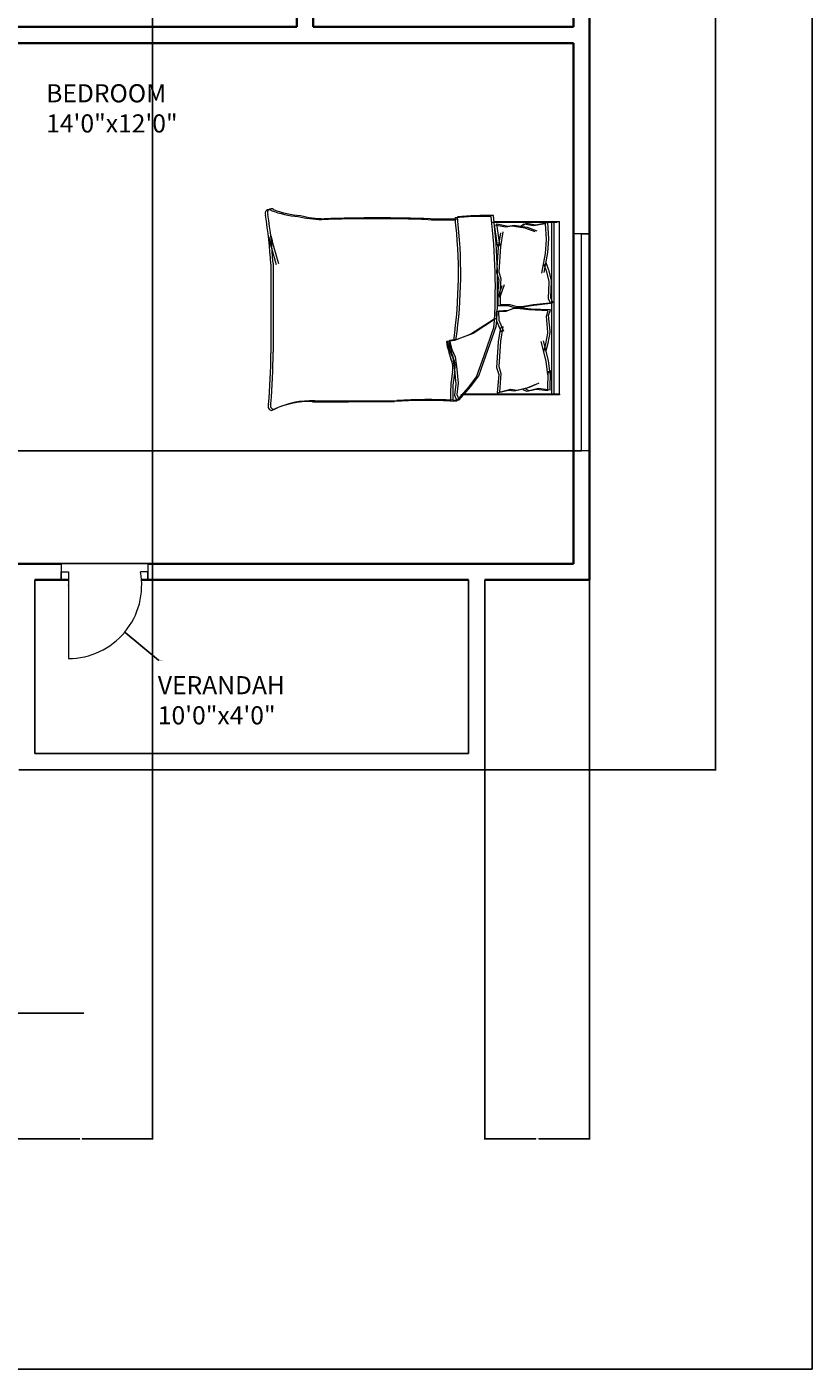
# Model space of a CAD drawing. Units: inches. Extents: x 1861 to 2564, y 1482 to 2317.
# Tile 3 of 11: x 2347 to 2564, y 1482 to 1853. Entities that reach past the tile are written whole.
import ezdxf

# ---------------------------------------------------------------- set-up
doc = ezdxf.new("R2010")
doc.units = ezdxf.units.IN
for name, color, linetype, lineweight in [('A-ANNO-DIMS', 2, 'Continuous', 18), ('A-ANNO-TTLB', 7, 'Continuous', 25), ('A-AREA-IDEN', 7, 'Continuous', 18), ('A-DOOR', 3, 'Continuous', 18), ('A-FLOR-EDGE', 7, 'Continuous', 25), ('A-FURN', 8, 'Continuous', 13), ('A-GLAZ', 4, 'Continuous', 18), ('A-WALL', 7, 'Continuous', 35)]:
    doc.layers.add(name, color=color, linetype=linetype, lineweight=lineweight)
doc.styles.get("Standard").update_dxf_attribs({"font": 'arial.ttf'})
doc.dimstyles.get("Standard").update_dxf_attribs({"dimtxt": 0.18, "dimasz": 0.18, "dimexe": 0.18, "dimexo": 0.0625, "dimgap": 0.09, "dimtad": 0, "dimtih": 1, "dimtoh": 1, "dimdec": 4, "dimzin": 0, "dimdsep": 46, "dimtxsty": 'Standard', "dimcen": 0.09, "dimadec": 0, "dimazin": 0, "dimtfac": 1, "dimtdec": 4, "dimtofl": 0, "dimtmove": 0, "dimatfit": 3, "dimfxl": 1, "dimtolj": 1, "dimtzin": 0, "dimarcsym": 0})

# ---------------------------------------------------------------- blocks, each defined once
blk = doc.blocks.new('WIN-60IN')
for p, q in [((0, 4.5), (0, 0)), ((60, 2.25), (60, 4.5)), ((60, 4.5), (60, 0)), ((0, 0), (0, 2.25)), ((0, 2.25), (60, 2.25))]:
    blk.add_line(p, q)
blk = doc.blocks.new('BED-DOUBLE')
for p, q in [((3.48, 63.34), (3.48, 81.45)), ((3.48, 63.34), (3.48, 81.45)), ((51.27, 81.45), (3.48, 81.45)), ((3.48, 79.91), (51.27, 79.91)), ((3.48, 79.91), (51.27, 79.91)), ((3.7, 62.7), (3.7, 80.81)), ((3.7, 62.7), (3.7, 80.81)), ((3.7, 79.27), (51.49, 79.27)), ((3.7, 79.27), (51.49, 79.27)), ((3.9, 78.11), (8.18, 78.44)), ((3.9, 78.11), (8.18, 78.44)), ((3.9, 78.13), (4.47, 74.95)), ((3.9, 78.13), (4.47, 74.95)), ((8.18, 78.44), (8.29, 78.42)), ((8.18, 78.44), (8.29, 78.42)), ((8.29, 78.42), (12.11, 78.13)), ((8.29, 78.42), (12.11, 78.13)), ((12.11, 78.13), (17.6, 77.12)), ((12.11, 78.13), (17.6, 77.12)), ((14.86, 77.7), (16.88, 78.42)), ((14.86, 77.7), (16.88, 78.42)), ((16.88, 78.42), (19.77, 79.14)), ((16.88, 78.42), (19.77, 79.14)), ((17.11, 77.78), (20, 78.5)), ((17.11, 77.78), (20, 78.5)), ((19.77, 79.14), (20.09, 79.14)), ((19.77, 79.14), (20.09, 79.14)), ((20, 78.5), (20.32, 78.5)), ((20, 78.5), (20.32, 78.5)), ((20.09, 79.14), (24.54, 79)), ((20.09, 79.14), (24.54, 79)), ((20.32, 78.5), (24.77, 78.36)), ((20.32, 78.5), (24.77, 78.36)), ((24.54, 79), (25.98, 79.58)), ((24.54, 79), (25.98, 79.58)), ((24.77, 78.36), (26.21, 78.94)), ((24.77, 78.36), (26.21, 78.94)), ((25.98, 79.58), (26.56, 74.23)), ((25.98, 79.58), (26.56, 74.23)), ((26.21, 78.94), (26.79, 73.59)), ((26.21, 78.94), (26.79, 73.59)), ((27.98, 78.95), (27.73, 73.58)), ((27.98, 78.95), (27.73, 73.58)), ((28.21, 78.31), (27.96, 72.94)), ((28.21, 78.31), (27.96, 72.94)), ((29.46, 78.47), (27.98, 78.95)), ((29.46, 78.47), (27.98, 78.95)), ((29.69, 77.83), (28.21, 78.31)), ((29.68, 77.83), (28.21, 78.31)), ((33.88, 78.89), (29.46, 78.47)), ((33.88, 78.89), (29.46, 78.47)), ((34.11, 78.25), (29.68, 77.83)), ((34.11, 78.25), (29.69, 77.83)), ((34.21, 78.91), (33.88, 78.89)), ((34.21, 78.91), (33.88, 78.89)), ((34.43, 78.27), (34.11, 78.25)), ((34.43, 78.27), (34.11, 78.25)), ((37.14, 78.37), (34.21, 78.91)), ((37.14, 78.37), (34.21, 78.91)), ((37.36, 77.73), (34.43, 78.27)), ((37.36, 77.73), (34.43, 78.27)), ((41.92, 78.38), (36.5, 77.02)), ((41.92, 78.38), (36.5, 77.02)), ((39.2, 77.77), (37.14, 78.37)), ((39.2, 77.77), (37.14, 78.37)), ((45.71, 78.9), (41.92, 78.38)), ((45.71, 78.9), (41.92, 78.38)), ((45.94, 78.26), (42.14, 77.74)), ((45.94, 78.26), (42.14, 77.74)), ((50.11, 78.89), (44.71, 78.99)), ((44.71, 78.99), (45.71, 78.9)), ((50.11, 78.89), (44.71, 78.99)), ((44.71, 78.99), (45.71, 78.9)), ((50.34, 78.25), (44.94, 78.35)), ((44.94, 78.35), (45.94, 78.26)), ((50.34, 78.25), (44.94, 78.35)), ((44.94, 78.35), (45.94, 78.26)), ((50.11, 78.89), (49.73, 75.68)), ((50.11, 78.89), (49.73, 75.68)), ((50.34, 78.25), (49.96, 75.04)), ((50.34, 78.25), (49.96, 75.04)), ((51.27, 81.45), (51.27, 54.84)), ((51.27, 81.45), (51.27, 54.84)), ((51.27, 81.45), (51.49, 81.45)), ((51.49, 81.45), (51.49, 80.81)), ((51.49, 80.81), (51.49, 54.2)), ((51.49, 80.81), (51.49, 54.2)), ((4.47, 74.95), (4.04, 72.35)), ((4.47, 74.95), (4.04, 72.35)), ((4.12, 77.49), (4.7, 74.31)), ((4.12, 77.49), (4.7, 74.31)), ((4.13, 77.47), (8.41, 77.8)), ((4.13, 77.47), (8.41, 77.8)), ((4.7, 74.31), (4.27, 71.71)), ((4.7, 74.31), (4.27, 71.71)), ((5.05, 72.49), (6.06, 75.24)), ((5.05, 72.49), (6.06, 75.24)), ((5.28, 71.85), (6.29, 74.6)), ((5.28, 71.85), (6.29, 74.6)), ((8.41, 77.8), (8.51, 77.78)), ((8.41, 77.8), (8.51, 77.78)), ((8.51, 77.78), (12.34, 77.49)), ((8.51, 77.78), (12.34, 77.49)), ((12.34, 77.49), (17.83, 76.48)), ((12.34, 77.49), (17.83, 76.48)), ((15.08, 77.06), (17.11, 77.78)), ((15.08, 77.06), (17.11, 77.78)), ((42.14, 77.74), (36.72, 76.38)), ((42.14, 77.74), (36.72, 76.38)), ((39.43, 77.13), (37.36, 77.73)), ((39.43, 77.13), (37.36, 77.73)), ((49.31, 73.19), (48.13, 75.87)), ((49.31, 73.19), (48.13, 75.87)), ((49.54, 72.55), (48.36, 75.23)), ((49.54, 72.55), (48.36, 75.23)), ((49.73, 75.68), (50.33, 73.11)), ((49.73, 75.68), (50.33, 73.11)), ((49.96, 75.04), (50.56, 72.47)), ((49.96, 75.04), (50.56, 72.47)), ((4.04, 72.35), (4.62, 71.33)), ((4.04, 72.35), (4.62, 71.33)), ((4.27, 71.71), (4.85, 70.69)), ((4.27, 71.71), (4.85, 70.69)), ((4.47, 68.88), (5.05, 72.49)), ((4.47, 68.88), (5.05, 72.49)), ((4.7, 68.24), (5.28, 71.85)), ((4.7, 68.24), (5.28, 71.85)), ((26.56, 74.23), (27.14, 71.04)), ((26.56, 74.23), (27.14, 71.04)), ((26.79, 73.59), (27.37, 70.41)), ((26.79, 73.59), (27.37, 70.41)), ((27.14, 71.04), (27.14, 69.74)), ((27.14, 71.04), (27.14, 69.74)), ((27.73, 73.58), (27.36, 70.37)), ((27.73, 73.58), (27.36, 70.37)), ((27.96, 72.94), (27.58, 69.73)), ((27.96, 72.94), (27.58, 69.73)), ((50.11, 69.62), (49.31, 73.19)), ((50.11, 69.62), (49.31, 73.19)), ((50.34, 68.98), (49.54, 72.55)), ((50.34, 68.98), (49.54, 72.55)), ((50.33, 73.11), (49.82, 72.06)), ((50.33, 73.11), (49.82, 72.06)), ((50.56, 72.47), (50.04, 71.42)), ((50.56, 72.47), (50.04, 71.42)), ((4.18, 64.1), (4.76, 67.29)), ((4.18, 64.1), (4.76, 67.29)), ((4.76, 67.29), (4.47, 68.88)), ((4.76, 67.29), (4.47, 68.88)), ((4.99, 66.65), (4.7, 68.24)), ((4.99, 66.65), (4.7, 68.24)), ((27.14, 69.74), (26.56, 67.86)), ((27.14, 69.74), (26.56, 67.86)), ((26.56, 67.86), (26.56, 65.18)), ((26.56, 67.86), (26.56, 65.18)), ((27.37, 69.1), (26.79, 67.22)), ((27.37, 69.1), (26.79, 67.22)), ((26.79, 67.22), (26.79, 64.54)), ((26.79, 67.22), (26.79, 64.54)), ((27.36, 70.37), (27.44, 69.07)), ((27.36, 70.37), (27.44, 69.07)), ((27.37, 70.41), (27.37, 69.1)), ((27.37, 70.41), (27.37, 69.1)), ((27.44, 69.07), (28.13, 67.23)), ((27.44, 69.07), (28.13, 67.23)), ((27.58, 69.73), (27.67, 68.43)), ((27.58, 69.73), (27.67, 68.43)), ((27.67, 68.43), (28.36, 66.59)), ((27.67, 68.43), (28.36, 66.59)), ((28.13, 67.23), (28.3, 64.55)), ((28.13, 67.23), (28.3, 64.55)), ((49.92, 68.01), (50.11, 69.62)), ((49.92, 68.01), (50.11, 69.62)), ((50.7, 64.87), (49.92, 68.01)), ((50.7, 64.87), (49.92, 68.01)), ((50.15, 67.37), (50.34, 68.98)), ((50.15, 67.37), (50.34, 68.98)), ((50.93, 64.23), (50.15, 67.37)), ((50.93, 64.23), (50.15, 67.37)), ((9.28, 64.83), (4.18, 64.1)), ((9.28, 64.83), (4.18, 64.1)), ((4.41, 63.46), (4.99, 66.65)), ((4.41, 63.46), (4.99, 66.65)), ((9.51, 64.19), (4.41, 63.46)), ((9.51, 64.19), (4.41, 63.46)), ((6.38, 65.82), (10.41, 65.15)), ((6.38, 65.82), (10.41, 65.15)), ((6.61, 65.18), (10.64, 64.51)), ((6.61, 65.18), (10.64, 64.51)), ((10.41, 65.15), (9.28, 64.83)), ((10.41, 65.15), (9.28, 64.83)), ((10.64, 64.51), (9.51, 64.19)), ((10.64, 64.51), (9.51, 64.19)), ((10.41, 65.15), (17.42, 64.72)), ((10.41, 65.15), (17.42, 64.72)), ((10.64, 64.51), (17.65, 64.08)), ((10.64, 64.51), (17.65, 64.08)), ((17.42, 64.72), (19.38, 65.28)), ((17.42, 64.72), (19.38, 65.28)), ((17.65, 64.08), (19.61, 64.64)), ((17.65, 64.08), (19.61, 64.64)), ((19.38, 65.28), (24.52, 64.87)), ((19.38, 65.28), (24.52, 64.87)), ((19.61, 64.64), (24.75, 64.23)), ((19.61, 64.64), (24.74, 64.23)), ((24.1, 65.18), (20.96, 66.27)), ((24.1, 65.18), (20.96, 66.27)), ((24.33, 64.54), (21.19, 65.63)), ((24.33, 64.54), (21.19, 65.63)), ((26.56, 65.18), (24.1, 65.18)), ((26.56, 65.18), (24.1, 65.18)), ((26.79, 64.54), (24.33, 64.54)), ((26.79, 64.54), (24.33, 64.54)), ((28.3, 64.55), (30.75, 64.71)), ((28.3, 64.55), (30.75, 64.71)), ((28.36, 66.59), (28.53, 63.91)), ((28.36, 66.59), (28.53, 63.91)), ((28.53, 63.91), (30.98, 64.07)), ((28.53, 63.91), (30.98, 64.07)), ((30.26, 64.06), (34.45, 57.57)), ((30.26, 64.06), (34.45, 57.57)), ((30.49, 63.42), (34.68, 56.93)), ((30.49, 63.42), (34.68, 56.93)), ((30.75, 64.71), (33.82, 65.99)), ((30.75, 64.71), (33.82, 65.99)), ((30.98, 64.07), (34.05, 65.35)), ((30.98, 64.07), (34.05, 65.35)), ((40.65, 61.13), (32.31, 64.06)), ((40.64, 61.13), (32.31, 64.06)), ((40.87, 60.49), (32.54, 63.42)), ((40.87, 60.49), (32.54, 63.42)), ((32.56, 65.82), (36.6, 65.15)), ((32.57, 65.82), (36.6, 65.15)), ((32.79, 65.18), (36.83, 64.51)), ((32.79, 65.18), (36.83, 64.51)), ((36.6, 65.15), (43.61, 64.72)), ((36.6, 65.15), (43.61, 64.72)), ((36.83, 64.51), (43.84, 64.08)), ((36.83, 64.51), (43.84, 64.08)), ((43.61, 64.72), (45.57, 65.28)), ((43.61, 64.72), (45.57, 65.28)), ((43.84, 64.08), (45.8, 64.64)), ((43.84, 64.08), (45.8, 64.64)), ((45.57, 65.28), (50.7, 64.87)), ((45.57, 65.28), (50.7, 64.87)), ((45.8, 64.64), (50.93, 64.23)), ((45.8, 64.64), (50.93, 64.23)), ((46.22, 59.12), (40.64, 61.13)), ((46.22, 59.12), (40.65, 61.13)), ((46.45, 58.48), (40.87, 60.49)), ((46.45, 58.48), (40.87, 60.49)), ((34.45, 57.57), (36.15, 53.08)), ((34.45, 57.57), (36.15, 53.08)), ((34.68, 56.93), (36.38, 52.44)), ((34.68, 56.93), (36.38, 52.44)), ((49.16, 56.95), (46.22, 59.12)), ((49.16, 56.95), (46.22, 59.12)), ((49.39, 56.31), (46.45, 58.48)), ((49.39, 56.31), (46.45, 58.48)), ((52.87, 53.7), (49.16, 56.95)), ((52.87, 53.7), (49.16, 56.95)), ((53.1, 53.06), (49.39, 56.31)), ((53.1, 53.06), (49.39, 56.31)), ((36.15, 53.08), (36.46, 51.07)), ((36.15, 53.08), (36.46, 51.07)), ((36.38, 52.44), (36.69, 50.43)), ((36.38, 52.44), (36.69, 50.43)), ((38.94, 51.69), (40.95, 52.62)), ((38.94, 51.69), (40.95, 52.62)), ((40.95, 52.62), (44.36, 53.08)), ((40.95, 52.62), (44.36, 53.08)), ((41.18, 51.98), (44.59, 52.44)), ((41.18, 51.98), (44.59, 52.44)), ((44.36, 53.08), (48.23, 53.39)), ((44.36, 53.08), (48.23, 53.39)), ((44.59, 52.44), (48.46, 52.75)), ((44.59, 52.44), (48.46, 52.75)), ((48.23, 53.39), (51.33, 53.08)), ((48.23, 53.39), (51.33, 53.08)), ((48.46, 52.75), (51.56, 52.44)), ((48.46, 52.75), (51.56, 52.44)), ((51.33, 53.08), (52.87, 53.7)), ((51.33, 53.08), (52.87, 53.7)), ((51.56, 52.44), (53.1, 53.06)), ((51.56, 52.44), (53.1, 53.06)), ((52.95, 51.95), (52.87, 53.7, 3.87)), ((52.95, 51.95), (52.87, 53.7, 3.87)), ((53.18, 51.32), (53.1, 53.06, 3.87)), ((53.18, 51.32), (53.1, 53.06, 3.87)), ((36.46, 51.07), (38.94, 51.69)), ((36.46, 51.07), (38.94, 51.69)), ((36.69, 50.43), (39.17, 51.05)), ((36.69, 50.43), (39.17, 51.05)), ((39.17, 51.05), (41.18, 51.98)), ((39.17, 51.05), (41.18, 51.98)), ((15.06, 2.2), (39.68, 2.2)), ((15.06, 2.2), (39.68, 2.2)), ((15.29, 1.56), (39.91, 1.56)), ((15.29, 1.56), (39.91, 1.56))]:
    blk.add_line(p, q)
for centre, radius, start, end in [((85.16, 61.35), 83.31, 178.7218, 185.604), ((85.16, 61.35), 83.31, 178.7218, 185.604), ((21.36, -100.61), 164.97, 86.0865, 96.7821), ((21.36, -100.61), 164.97, 86.0865, 96.7821), ((21.59, -101.25), 164.97, 86.0865, 96.7821), ((21.59, -101.25), 164.97, 86.0865, 96.7821), ((85.39, 60.71), 83.31, 178.7218, 185.604), ((85.39, 60.71), 83.31, 178.7218, 185.604), ((17.76, -74.87), 129.02, 81.7845, 96.9006), ((17.76, -74.87), 129.02, 81.7845, 96.9006), ((17.99, -75.51), 129.02, 81.7845, 96.9006), ((17.98, -75.51), 129.02, 81.7845, 96.9006), ((-167.31, 50.27), 170.11, 358.4762, 1.0082), ((-167.31, 50.27), 170.11, 358.4762, 1.0082), ((-167.08, 49.63), 170.11, 358.4762, 1.0082), ((-167.08, 49.63), 170.11, 358.4762, 1.0082), ((31.15, 79.96), 29.65, 280.6617, 289.8806), ((31.15, 79.96), 29.65, 280.6617, 289.8806), ((43.74, 46.38), 6.22, 78.6608, 113.7384), ((43.74, 46.38), 6.22, 78.6608, 113.7384), ((51.33, 88.1), 36.18, 259.8763, 272.5657), ((51.33, 88.1), 36.18, 259.8763, 272.5657), ((36.64, 51.01), 0.185, 160.2464, 271.1377), ((36.64, 51.01), 0.185, 160.2464, 271.1377), ((36.87, 50.37), 0.185, 160.2464, 271.1377), ((36.87, 50.37), 0.185, 160.2464, 271.1377), ((31.38, 79.32), 29.65, 280.6617, 289.8806), ((31.38, 79.32), 29.65, 280.6617, 289.8806), ((43.97, 45.74), 6.22, 78.6608, 113.7384), ((43.97, 45.74), 6.22, 78.6608, 113.7384), ((51.56, 87.46), 36.18, 259.8763, 272.5657), ((51.56, 87.46), 36.18, 259.8763, 272.5657), ((182.27, 45.13), 129.5, 176.9791, 183.8365), ((182.27, 45.13), 129.5, 176.9791, 183.8365), ((182.5, 44.49), 129.5, 176.9791, 183.8365), ((182.49, 44.49), 129.5, 176.9791, 183.8365), ((484.82, 30.83), 482.31, 178.2277, 181.7185), ((484.82, 30.83), 482.31, 178.2277, 181.7185), ((485.05, 30.19), 482.31, 178.2277, 181.7185), ((485.05, 30.19), 482.31, 178.2277, 181.7185), ((-4508.74, 13.62), 4561.86, 0.00217, 0.28689), ((-4508.74, 13.62), 4561.86, 0.00217, 0.28689), ((-4508.51, 12.98), 4561.86, 0.00217, 0.28689), ((-4508.51, 12.98), 4561.86, 0.00217, 0.28689), ((-26.9, 16.93), 29.63, 346.0648, 358.9113), ((-26.9, 16.93), 29.63, 346.0648, 358.9113), ((-26.67, 16.29), 29.63, 346.0648, 358.9113), ((-26.67, 16.29), 29.63, 346.0648, 358.9113), ((76.16, 12.78), 23.07, 177.4714, 206.4681), ((76.16, 12.78), 23.07, 177.4714, 206.4681), ((76.39, 12.14), 23.07, 177.4714, 206.4681), ((76.39, 12.14), 23.07, 177.4714, 206.4681), ((-21.66, 11.17), 23.56, 337.9751, 356.652), ((-21.66, 11.17), 23.56, 337.9751, 356.652), ((-21.43, 10.53), 23.56, 337.9751, 356.652), ((-21.43, 10.53), 23.56, 337.9751, 356.652), ((-17.22, 105.16), 106.46, 283.3832, 287.7053), ((-17.22, 105.16), 106.46, 283.3832, 287.7053), ((1.09, 1.73), 1.09, 146.1736, 293.4781), ((1.09, 1.73), 1.09, 146.1736, 293.4781), ((1.32, 1.09), 1.09, 146.1736, 293.4781), ((1.32, 1.09), 1.09, 146.1736, 293.4781), ((21.43, -119.39), 121.76, 92.9958, 99.4091), ((21.43, -119.39), 121.76, 92.9958, 99.4091), ((21.66, -120.03), 121.76, 92.9958, 99.4091), ((21.66, -120.03), 121.76, 92.9958, 99.4091), ((-16.99, 104.52), 106.46, 283.3832, 287.7053), ((-16.99, 104.52), 106.46, 283.3832, 287.7053), ((41.15, -130.83), 133.04, 84.4998, 90.6351), ((41.15, -130.83), 133.04, 84.4998, 90.6351), ((41.38, -131.47), 133.04, 84.4998, 90.6351), ((41.38, -131.47), 133.04, 84.4998, 90.6351), ((54.41, 2.58), 1.1, 242.6588, 356.02), ((54.41, 2.58), 1.1, 242.6588, 356.02), ((54.64, 1.94), 1.1, 242.6588, 356.02), ((54.64, 1.94), 1.1, 242.6588, 356.02)]:
    blk.add_arc(centre, radius, start, end)
blk = doc.blocks.new('*D38')
at = {"layer": 'A-ANNO-DIMS', "color": 0, "lineweight": -2, "transparency": 16777216}
for p, q in [((2341.74, 2250.82), (2341.74, 1545.6)), ((2381.24, 2250.82), (2381.24, 1545.6)), ((2341.92, 1545.78), (2361.16, 1545.78)), ((2381.06, 1545.78), (2361.81, 1545.78))]:
    blk.add_line(p, q, dxfattribs=at)
at = {"layer": 'A-ANNO-DIMS', "color": 0, "transparency": 16777216}
for points in [[(2341.92, 1545.81), (2341.92, 1545.75), (2341.74, 1545.78)], [(2381.06, 1545.81), (2381.06, 1545.75), (2381.24, 1545.78)]]:
    blk.add_solid(points, dxfattribs=at)
at = {"layer": 'Defpoints', "color": 0, "transparency": 16777216}
for p in [(2341.74, 2250.89), (2381.24, 2250.89), (2381.24, 1545.78)]:
    blk.add_point(p, dxfattribs=at)
at = {"layer": 'A-ANNO-DIMS', "color": 0, "transparency": 16777216, "insert": (2361.49, 1545.78), "char_height": 0.18, "attachment_point": 5}
blk.add_mtext('\\A1;39.5', dxfattribs=at)
blk = doc.blocks.new('*D45')
at = {"layer": 'A-ANNO-DIMS', "color": 0, "lineweight": -2, "transparency": 16777216}
for p, q in [((2502.3, 2255.39), (2537.22, 2255.39)), ((2537.04, 2255.21), (2537.04, 1951.82)), ((2537.04, 1648.07), (2537.04, 1951.45)), ((2473.32, 1647.89), (2537.22, 1647.89))]:
    blk.add_line(p, q, dxfattribs=at)
at = {"layer": 'A-ANNO-DIMS', "color": 0, "transparency": 16777216}
for points in [[(2537.01, 2255.21), (2537.07, 2255.21), (2537.04, 2255.39)], [(2537.01, 1648.07), (2537.07, 1648.07), (2537.04, 1647.89)]]:
    blk.add_solid(points, dxfattribs=at)
at = {"layer": 'Defpoints', "color": 0, "transparency": 16777216}
for p in [(2502.24, 2255.39), (2537.04, 2255.39), (2473.26, 1647.89)]:
    blk.add_point(p, dxfattribs=at)
at = {"layer": 'A-ANNO-DIMS', "color": 0, "transparency": 16777216, "insert": (2537.04, 1951.64), "char_height": 0.18, "attachment_point": 5}
blk.add_mtext('\\A1;607.5', dxfattribs=at)
blk = doc.blocks.new('*D49')
at = {"layer": 'A-ANNO-DIMS', "color": 0, "lineweight": -2, "transparency": 16777216}
for p, q in [((2502.24, 1700.32), (2502.24, 1545.6)), ((2473.26, 1647.82), (2473.26, 1545.6)), ((2473.44, 1545.78), (2487.35, 1545.78)), ((2502.06, 1545.78), (2488.15, 1545.78))]:
    blk.add_line(p, q, dxfattribs=at)
at = {"layer": 'A-ANNO-DIMS', "color": 0, "transparency": 16777216}
for points in [[(2473.44, 1545.81), (2473.44, 1545.75), (2473.26, 1545.78)], [(2502.06, 1545.81), (2502.06, 1545.75), (2502.24, 1545.78)]]:
    blk.add_solid(points, dxfattribs=at)
at = {"layer": 'Defpoints', "color": 0, "transparency": 16777216}
for p in [(2502.24, 1700.39), (2473.26, 1647.89), (2502.24, 1545.78)]:
    blk.add_point(p, dxfattribs=at)
at = {"layer": 'A-ANNO-DIMS', "color": 0, "transparency": 16777216, "insert": (2487.75, 1545.78), "char_height": 0.18, "attachment_point": 5}
blk.add_mtext('\\A1;28.98', dxfattribs=at)
blk = doc.blocks.new('*D67')
at = {"layer": 'A-ANNO-DIMS', "color": 0, "lineweight": -2, "transparency": 16777216}
for p, q in [((2497.68, 1736.13), (1892.76, 1736.13)), ((1892.94, 1735.95), (1892.94, 1720.69)), ((1892.94, 1705.07), (1892.94, 1720.32)), ((2497.68, 1704.89), (1892.76, 1704.89))]:
    blk.add_line(p, q, dxfattribs=at)
at = {"layer": 'A-ANNO-DIMS', "color": 0, "transparency": 16777216}
for points in [[(1892.91, 1735.95), (1892.97, 1735.95), (1892.94, 1736.13)], [(1892.91, 1705.07), (1892.97, 1705.07), (1892.94, 1704.89)]]:
    blk.add_solid(points, dxfattribs=at)
at = {"layer": 'Defpoints', "color": 0, "transparency": 16777216}
for p in [(1892.94, 1736.13), (2497.74, 1736.13), (2497.74, 1704.89)]:
    blk.add_point(p, dxfattribs=at)
at = {"layer": 'A-ANNO-DIMS', "color": 0, "transparency": 16777216, "insert": (1892.94, 1720.51), "char_height": 0.18, "attachment_point": 5}
blk.add_mtext('\\A1;31.24', dxfattribs=at)
blk = doc.blocks.new('*D85')
at = {"layer": 'A-ANNO-DIMS', "color": 0, "lineweight": -2, "transparency": 16777216}
for p, q in [((2357.92, 1698.92), (2358.1, 1698.92)), ((2358.01, 1698.83), (2358.01, 1699.01)), ((2382.98, 1678.18), (2373.75, 1685.84)), ((2383.16, 1678.18), (2382.98, 1678.18))]:
    blk.add_line(p, q, dxfattribs=at)
at = {"layer": 'A-ANNO-DIMS', "color": 0, "transparency": 16777216}
blk.add_solid([(2373.77, 1685.86), (2373.73, 1685.82), (2373.61, 1685.96)], dxfattribs=at)
at = {"layer": 'Defpoints', "color": 0, "transparency": 16777216}
for p in [(2358.01, 1698.92), (2373.61, 1685.96)]:
    blk.add_point(p, dxfattribs=at)
at = {"layer": 'A-ANNO-DIMS', "color": 0, "transparency": 16777216, "insert": (2383.7, 1678.18), "char_height": 0.18, "attachment_point": 5}
blk.add_mtext('\\A1;R20.283', dxfattribs=at)

msp = doc.modelspace()

# ---------------------------------------------------------------- linework, layer by layer
at = {"layer": 'A-ANNO-TTLB'}
msp.add_line((2110.0229, 1580.5777), (2362.3195, 1580.5777), dxfattribs=at)
msp.add_lwpolyline([(1861.1332, 2316.6589), (2563.8077, 2316.6589), (2563.8077, 1482.0728), (1861.1332, 1482.0728)], close=True, dxfattribs=at)
at = {"layer": 'A-DOOR'}
for p, q in [((2356.0129, 1704.8854), (2356.0129, 1700.3854)), ((2379.953, 1704.8854), (2379.953, 1700.3854)), ((2356.0129, 1700.3854), (2356.0129, 1702.6354)), ((2356.0129, 1702.6354), (2358.0129, 1702.6354)), ((2358.0129, 1702.6354), (2358.0129, 1678.6354)), ((2379.953, 1702.6354), (2377.953, 1702.6354)), ((2379.953, 1700.3854), (2379.953, 1702.6354))]:
    msp.add_line(p, q, dxfattribs=at)
msp.add_arc((2358.0129, 1698.9189), 20.2835, 270, 10.557851, dxfattribs=at)
at = {"layer": 'A-FLOR-EDGE'}
for p, q in [((2348.7613, 1652.3854), (2348.7613, 1700.3854)), ((2468.7613, 1700.3854), (2468.7613, 1652.3854)), ((2473.2613, 1647.8854), (2473.2613, 1700.3854)), ((2468.7613, 1652.3854), (2348.7613, 1652.3854)), ((2344.2613, 1647.8854), (2468.7613, 1647.8854)), ((2468.7613, 1647.8854), (2473.2613, 1647.8854))]:
    msp.add_line(p, q, dxfattribs=at)
at = {"layer": 'A-WALL'}
for p, q in [((2502.2393, 2255.3854), (2502.2393, 1700.3854)), ((2421.2393, 1853.3854), (2421.2393, 1901.3854)), ((2425.7393, 1901.3854), (2425.7393, 1853.3854)), ((2497.7393, 1901.3854), (2497.7393, 1853.3854)), ((2421.2393, 1853.3854), (2318.8029, 1853.3854)), ((2497.7393, 1853.3854), (2425.7393, 1853.3854)), ((2316.9501, 1848.8854), (2497.7393, 1848.8854)), ((2497.7393, 1848.8854), (2329.7393, 1848.8854)), ((2497.7393, 1848.8854), (2497.7393, 1704.8854)), ((2356.0129, 1704.8854), (2329.7393, 1704.8854)), ((2497.7393, 1704.8854), (2379.953, 1704.8854)), ((2348.7613, 1700.3854), (2358.0129, 1700.3854)), ((2378.2433, 1700.3854), (2468.7613, 1700.3854)), ((2473.2613, 1700.3854), (2502.2393, 1700.3854))]:
    msp.add_line(p, q, dxfattribs=at)

# ---------------------------------------------------------------- block references
at = {"layer": 'A-FURN', "rotation": 270}
msp.add_blockref('BED-DOUBLE', (2412.4276, 1803.0388), dxfattribs=at)
at = {"layer": 'A-GLAZ', "extrusion": (0, 0, -1), "zscale": -1, "rotation": 90}
msp.add_blockref('WIN-60IN', (-2497.7439, 1736.127), dxfattribs=at)

# ---------------------------------------------------------------- texts
at = {"layer": 'A-AREA-IDEN', "char_height": 5, "attachment_point": 1}
for s, width, insert in [('BEDROOM\\P14\'0"x12\'0"', 156.051136, (2351.8669, 1837.503)), ('VERANDAH\\P10\'0"x4\'0"', 134.661698, (2382.7617, 1673.7728))]:
    msp.add_mtext_dynamic_manual_height_columns(s, width=width, gutter_width=12.5, heights=[0], dxfattribs=dict(at, insert=insert))

# ---------------------------------------------------------------- dimensions: what is measured, and where the dimension line sits
at = {"layer": 'A-ANNO-DIMS'}
for base, p1, p2, override, picture, middle in [((2537.0393, 2255.3854), (2473.2613, 1647.8854), (2502.2393, 2255.3854), {"dimdec": 1, "dimlfac": 1, "dimrnd": 0, "dimzin": 0, "dimdsep": 46, "dimlunit": 2}, '*D45', (2537.0393, 1951.6354)), ((1892.9393, 1736.1256), (2497.7393, 1704.8854), (2497.7393, 1736.1256), {"dimdec": 2, "dimlfac": 1, "dimrnd": 0, "dimzin": 0, "dimdsep": 46, "dimlunit": 2}, '*D67', (1892.9393, 1720.5055))]:
    dim = msp.add_linear_dim(base=base, p1=p1, p2=p2, angle=90, dimstyle='Standard', override=override, dxfattribs=at)
    dim.commit()
    dim.dimension.update_dxf_attribs({"geometry": picture, "text_midpoint": middle})
for base, p1, p2, override, picture, middle in [((2381.2368, 1545.7777), (2341.7393, 2250.8854), (2381.2368, 2250.8854), {"dimdec": 1, "dimlfac": 1, "dimrnd": 0, "dimzin": 0, "dimdsep": 46, "dimlunit": 2}, '*D38', (2361.488, 1545.7777)), ((2502.2393, 1545.7777), (2473.2613, 1647.8854), (2502.2393, 1700.3854), {"dimdec": 2, "dimlfac": 1, "dimrnd": 0, "dimzin": 0, "dimdsep": 46, "dimlunit": 2}, '*D49', (2487.7503, 1545.7777))]:
    dim = msp.add_linear_dim(base=base, p1=p1, p2=p2, dimstyle='Standard', override=override, dxfattribs=at)
    dim.commit()
    dim.dimension.update_dxf_attribs({"geometry": picture, "text_midpoint": middle})
dim = msp.add_radius_dim(center=(2358.01293, 1698.91889), mpoint=(2373.6143, 1685.95675), dimstyle='Standard', override={"dimdec": 3, "dimlfac": 1, "dimrnd": 0, "dimzin": 0, "dimdsep": 46, "dimlunit": 2}, dxfattribs=at)
dim.commit()
dim.dimension.update_dxf_attribs({"geometry": '*D85', "text_midpoint": (2383.70489, 1678.17946), "dimtype": 164})

doc.saveas('drawing.dxf')
